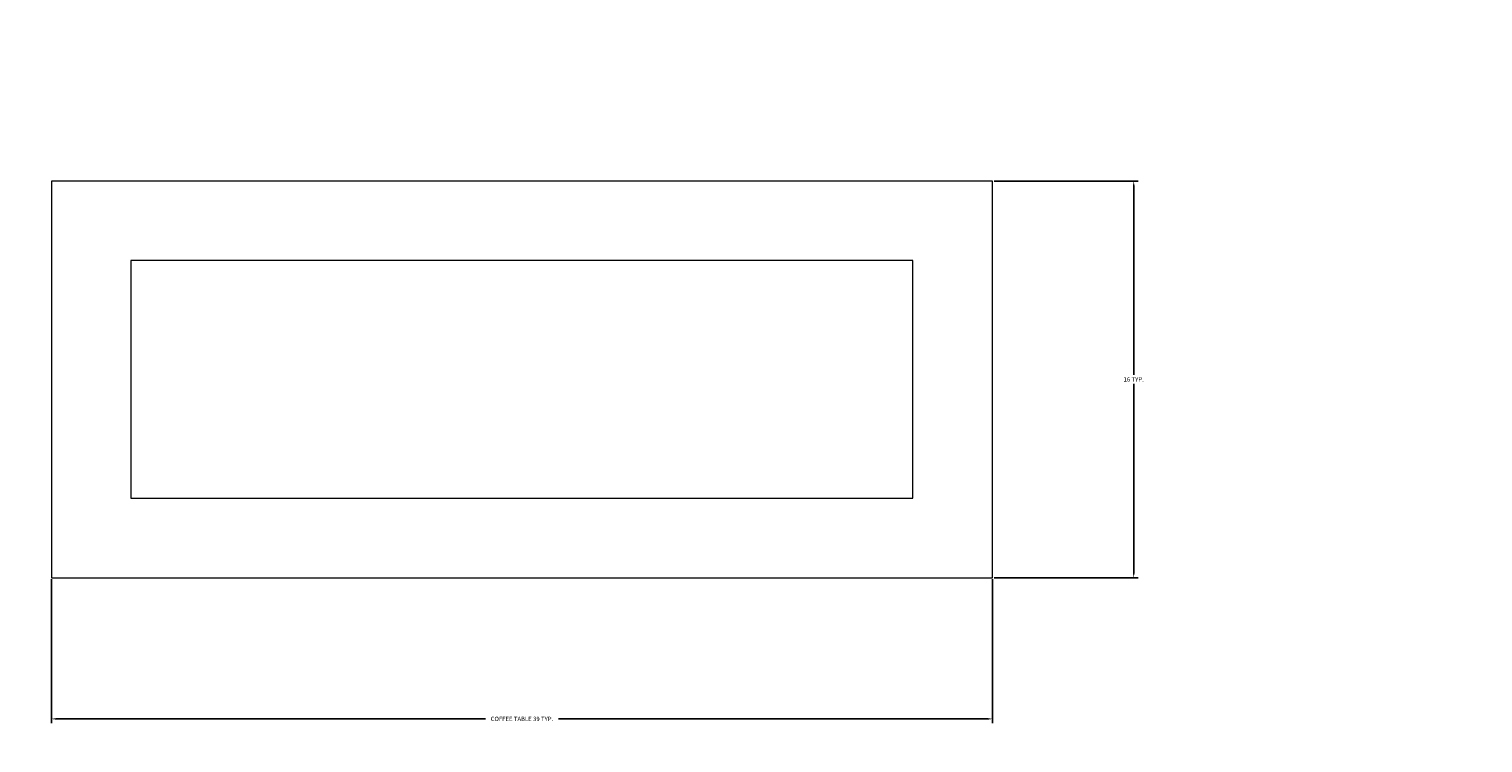
# Model space of a CAD drawing. Units: inches. Extents: x 1998 to 2588, y 1139 to 1977.
# Tile 127 of 134: x 2429 to 2489, y 1669 to 1698. Entities that reach past the tile are written whole.
import ezdxf

# ---------------------------------------------------------------- set-up
doc = ezdxf.new("R2010")
doc.units = ezdxf.units.IN
doc.layers.add('A-ANNO-DIMS', color=2, linetype='Continuous', lineweight=18)
doc.layers.add('FUR', color=21, linetype='Continuous', lineweight=18)
doc.styles.get("Standard").update_dxf_attribs({"font": 'arial.ttf'})
doc.dimstyles.get("Standard").update_dxf_attribs({"dimtxt": 0.18, "dimasz": 0.18, "dimexe": 0.18, "dimexo": 0.0625, "dimgap": 0.09, "dimtad": 0, "dimtih": 1, "dimtoh": 1, "dimdec": 4, "dimzin": 0, "dimdsep": 46, "dimtxsty": 'Standard', "dimcen": 0.09, "dimadec": 0, "dimazin": 0, "dimtfac": 1, "dimtdec": 4, "dimtofl": 0, "dimtmove": 0, "dimatfit": 3, "dimfxl": 1, "dimtolj": 1, "dimtzin": 0, "dimarcsym": 0})

# ---------------------------------------------------------------- blocks, each defined once
blk = doc.blocks.new('TABLE-COFFEE')
for points in [[(0, 0), (38.727, 0), (38.727, 16.33), (0, 16.33)], [(3.275, 3.276), (35.452, 3.276), (35.452, 13.055), (3.275, 13.055)]]:
    blk.add_lwpolyline(points, close=True)
blk = doc.blocks.new('*D15')
at = {"layer": 'A-ANNO-DIMS', "color": 0, "lineweight": -2, "transparency": 16777216}
for p, q in [((2429.857, 1675.587), (2429.857, 1669.661)), ((2468.584, 1675.587), (2468.584, 1669.661)), ((2430.037, 1669.841), (2447.715, 1669.841)), ((2468.404, 1669.841), (2450.725, 1669.841))]:
    blk.add_line(p, q, dxfattribs=at)
at = {"layer": 'A-ANNO-DIMS', "color": 0, "transparency": 16777216}
for points in [[(2430.037, 1669.871), (2430.037, 1669.811), (2429.857, 1669.841)], [(2468.404, 1669.871), (2468.404, 1669.811), (2468.584, 1669.841)]]:
    blk.add_solid(points, dxfattribs=at)
at = {"layer": 'Defpoints', "color": 0, "transparency": 16777216}
for p in [(2429.857, 1675.65), (2468.584, 1675.65), (2468.584, 1669.841)]:
    blk.add_point(p, dxfattribs=at)
at = {"layer": 'A-ANNO-DIMS', "color": 0, "transparency": 16777216, "insert": (2449.22, 1669.841), "char_height": 0.18, "attachment_point": 5}
blk.add_mtext('\\A1;COFFEE TABLE 39 TYP.', dxfattribs=at)
blk = doc.blocks.new('*D16')
at = {"layer": 'A-ANNO-DIMS', "color": 0, "lineweight": -2, "transparency": 16777216}
for p, q in [((2468.646, 1691.979), (2474.573, 1691.979)), ((2474.393, 1691.799), (2474.393, 1683.996)), ((2474.393, 1675.83), (2474.393, 1683.632)), ((2468.646, 1675.65), (2474.573, 1675.65))]:
    blk.add_line(p, q, dxfattribs=at)
at = {"layer": 'A-ANNO-DIMS', "color": 0, "transparency": 16777216}
for points in [[(2474.363, 1691.799), (2474.423, 1691.799), (2474.393, 1691.979)], [(2474.363, 1675.83), (2474.423, 1675.83), (2474.393, 1675.65)]]:
    blk.add_solid(points, dxfattribs=at)
at = {"layer": 'Defpoints', "color": 0, "transparency": 16777216}
for p in [(2468.584, 1691.979), (2474.393, 1691.979), (2468.584, 1675.65)]:
    blk.add_point(p, dxfattribs=at)
at = {"layer": 'A-ANNO-DIMS', "color": 0, "transparency": 16777216, "insert": (2474.393, 1683.814), "char_height": 0.18, "attachment_point": 5}
blk.add_mtext('\\A1;16 TYP.', dxfattribs=at)
blk = doc.blocks.new('*D24')
at = {"layer": 'A-ANNO-DIMS', "color": 0, "lineweight": -2, "transparency": 16777216}
for p, q in [((2398.535, 1911.232), (2588.309, 1911.232)), ((2588.129, 1911.052), (2588.129, 1570.164)), ((2588.129, 1228.912), (2588.129, 1569.8)), ((2527.535, 1228.732), (2588.309, 1228.732))]:
    blk.add_line(p, q, dxfattribs=at)
at = {"layer": 'A-ANNO-DIMS', "color": 0, "transparency": 16777216}
for points in [[(2588.099, 1911.052), (2588.159, 1911.052), (2588.129, 1911.232)], [(2588.099, 1228.912), (2588.159, 1228.912), (2588.129, 1228.732)]]:
    blk.add_solid(points, dxfattribs=at)
at = {"layer": 'Defpoints', "color": 0, "transparency": 16777216}
for p in [(2398.473, 1911.232), (2588.129, 1911.232), (2527.473, 1228.732)]:
    blk.add_point(p, dxfattribs=at)
at = {"layer": 'A-ANNO-DIMS', "color": 0, "transparency": 16777216, "insert": (2588.129, 1569.982), "char_height": 0.18, "attachment_point": 5}
blk.add_mtext('\\A1;682.5', dxfattribs=at)

msp = doc.modelspace()

# ---------------------------------------------------------------- block references
at = {"layer": 'FUR'}
msp.add_blockref('TABLE-COFFEE', (2429.8567, 1675.6492), dxfattribs=at)

# ---------------------------------------------------------------- dimensions: what is measured, and where the dimension line sits
at = {"layer": 'A-ANNO-DIMS'}
dim = msp.add_linear_dim(base=(2588.1286, 1911.2324), p1=(2527.4729, 1228.7324), p2=(2398.4729, 1911.2324), angle=90, dimstyle='Standard', override={"dimdec": 1, "dimlfac": 1, "dimrnd": 0, "dimzin": 0, "dimdsep": 46, "dimlunit": 2}, dxfattribs=at)
dim.commit()
dim.dimension.update_dxf_attribs({"geometry": '*D24', "text_midpoint": (2588.1286, 1569.9824)})
dim = msp.add_linear_dim(base=(2474.3928, 1691.9791), p1=(2468.5838, 1675.6496), p2=(2468.5838, 1691.9791), angle=90, text='<> TYP.', dimstyle='Standard', override={"dimdec": 0, "dimlfac": 1, "dimrnd": 0, "dimzin": 0, "dimdsep": 46, "dimlunit": 2}, dxfattribs=at)
dim.commit()
dim.dimension.update_dxf_attribs({"geometry": '*D16', "text_midpoint": (2474.3928, 1683.8143)})
dim = msp.add_linear_dim(base=(2468.5838, 1669.8405), p1=(2429.8567, 1675.6496), p2=(2468.5838, 1675.6496), text='COFFEE TABLE <> TYP.', dimstyle='Standard', override={"dimdec": 0, "dimlfac": 1, "dimrnd": 0, "dimzin": 0, "dimdsep": 46, "dimlunit": 2}, dxfattribs=at)
dim.commit()
dim.dimension.update_dxf_attribs({"geometry": '*D15', "text_midpoint": (2449.2202, 1669.8405)})

doc.saveas('drawing.dxf')
